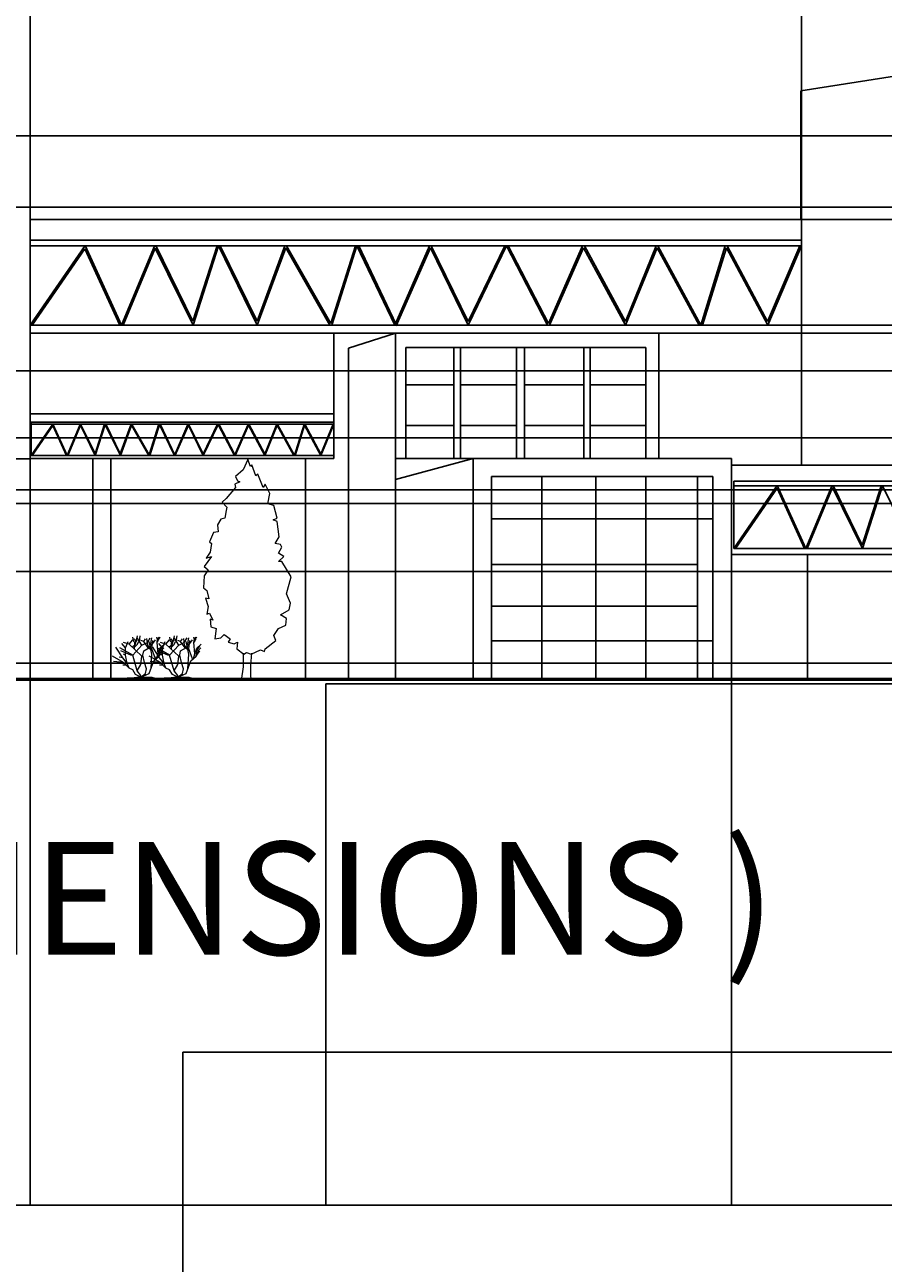
# Model space of a CAD drawing. Units: inches. Extents: x -32109 to 33221, y -19197 to 7608.
# Tile 18 of 25: x 6939 to 12337, y -5795 to 1998. Entities that reach past the tile are written whole.
import ezdxf

# ---------------------------------------------------------------- set-up
doc = ezdxf.new("R2010")
doc.units = ezdxf.units.IN
doc.header["$MEASUREMENT"] = 0
for name, color, linetype, lineweight in [('A-ANNO-DIMS', 2, 'Continuous', 18), ('A-ANNO-TEXT', 7, 'Continuous', 25), ('A-ELEV', 7, 'Continuous', 25), ('L-PLNT', 3, 'Continuous', 13)]:
    doc.layers.add(name, color=color, linetype=linetype, lineweight=lineweight)
doc.styles.get("Standard").update_dxf_attribs({"font": 'arial.ttf'})
doc.dimstyles.get("Standard").update_dxf_attribs({"dimtxt": 0.18, "dimasz": 0.18, "dimexe": 0.18, "dimexo": 0.0625, "dimgap": 0.09, "dimtad": 0, "dimtih": 1, "dimtoh": 1, "dimdec": 4, "dimzin": 0, "dimdsep": 46, "dimtxsty": 'Standard', "dimcen": 0.09, "dimadec": 0, "dimazin": 0, "dimtfac": 1, "dimtdec": 4, "dimtofl": 0, "dimtmove": 0, "dimatfit": 3, "dimfxl": 1, "dimtolj": 1, "dimtzin": 0, "dimarcsym": 0})

# ---------------------------------------------------------------- blocks, each defined once
blk = doc.blocks.new('*U2')
blk.add_lwpolyline([(-2.754, 191.699), (-6.78, 182.851), (-13.682, 176.953), (-11.956, 173.266), (-9.656, 172.529), (-14.257, 170.317), (-13.682, 167.368), (-21.733, 157.783), (-25.184, 154.834), (-21.158, 150.41), (-21.733, 147.461), (-22.884, 140.825), (-26.334, 140.087), (-29.21, 134.926), (-28.635, 129.028), (-32.661, 128.291), (-36.111, 120.18), (-34.386, 118.706), (-35.536, 111.333), (-38.987, 106.171), (-34.386, 107.646), (-40.712, 98.798), (-37.261, 95.849), (-40.712, 90.688), (-41.287, 80.366), (-38.412, 78.154), (-36.686, 70.781), (-39.562, 71.518), (-37.261, 64.145), (-38.412, 57.509), (-36.111, 58.247), (-33.236, 52.348), (-35.536, 53.086), (-34.961, 46.45), (-30.36, 44.975), (-31.51, 36.128), (-26.334, 36.865), (-23.459, 39.814), (-18.283, 36.128), (-20.008, 33.178), (-14.832, 31.704), (-11.956, 33.178), (-12.531, 27.28), (-6.205, 22.856), (-3.905, 24.331), (0.121, 22.856), (8.173, 26.543), (11.624, 25.068), (12.199, 27.28), (21.4, 34.653), (19.675, 39.077), (23.701, 44.975), (30.027, 47.924), (30.602, 53.823), (25.426, 56.772), (32.903, 61.196), (34.053, 67.094), (30.602, 75.205), (34.628, 89.951), (26.576, 103.222), (23.701, 103.222), (28.302, 107.646), (23.701, 110.595), (26.576, 115.756), (25.426, 117.968), (20.825, 118.706), (24.276, 124.604), (22.551, 137.876), (19.1, 139.35), (22.551, 140.825), (19.675, 151.884), (14.499, 153.359), (16.224, 162.207), (12.199, 170.317), (10.473, 167.368), (5.872, 179.165), (4.147, 177.69), (0.696, 187.275), (-0.454, 185.8)], close=True)
for points in [[(-6.813, 23.669), (-6.813, 11.669), (-8.627, 0)], [(0.387, 23.669), (-0.576, 13.271), (-0.576, 3.686), (0, 0)]]:
    blk.add_lwpolyline(points)
blk = doc.blocks.new('*U3')
for p, q in [((-16.8, 16.32), (-15.36, 19.68)), ((-14.88, 18.24), (-12.96, 20.64)), ((-12.471, 19.775), (-12.898, 22.044)), ((-11.677, 19.071), (-12.471, 19.775)), ((-11.28, 19.619), (-12.104, 21.184)), ((-11.921, 18.836), (-10.64, 20.401)), ((-11.433, 18.289), (-10.457, 22.749)), ((-10.579, 18.054), (-9.846, 19.697)), ((-8.16, 17.76), (-10.56, 21.6)), ((-9.48, 19.775), (-8.992, 22.592)), ((-7.2, 19.68), (-8.64, 20.16)), ((-7.2, 19.68), (-6.24, 21.12)), ((-4.8, 16.32), (-7.2, 19.68)), ((-5.086, 17.741), (-5.513, 21.34)), ((-5.28, 19.2), (-3.84, 21.6)), ((-2.88, 12.96), (-4.32, 19.68)), ((-3.84, 16.8), (-0.96, 20.64)), ((-3.377, 18.602), (-2.888, 21.575)), ((-2.88, 15.84), (-2.4, 20.16)), ((-0.508, 21.888), (-0.081, 20.558)), ((-0.203, 19.149), (0.102, 21.34)), ((-0.142, 19.384), (0.59, 20.401)), ((-0.02, 20.01), (0.896, 21.105)), ((0.041, 20.714), (1.384, 22.044)), ((0.102, 21.34), (0.835, 21.888)), ((-18.24, 11.04), (-21.755, 16.655)), ((-12.96, 12.48), (-19.68, 16.32)), ((-13.92, 12.48), (-19.2, 14.88)), ((-16.8, 16.32), (-18.72, 18.72)), ((-14.88, 18.24), (-17.76, 19.2)), ((-16.8, 12.48), (-16.8, 16.32)), ((-8.16, 12), (-14.88, 18.24)), ((-13.325, 16.724), (-11.433, 18.289)), ((-12.96, 12.48), (-8.16, 17.76)), ((-12.043, 15.628), (-11.921, 18.836)), ((-11.982, 16.802), (-10.579, 18.054)), ((-8.16, 17.76), (-5.28, 19.2)), ((-7.68, 12.48), (-7.2, 14.88)), ((-7.2, 14.88), (-3.84, 16.8)), ((-3.377, 15.315), (-5.086, 17.819)), ((-2.766, 16.802), (-3.377, 18.602)), ((-0.96, 10.56), (-2.88, 15.84)), ((-0.48, 10.8), (0.346, 13.203)), ((0.346, 13.203), (-0.203, 19.149)), ((0.346, 13.203), (1.323, 16.254)), ((0.96, 12), (1.44, 15.36)), ((0.96, 12), (2.88, 14.88)), ((1.323, 16.254), (3.642, 18.289)), ((1.44, 15.36), (2.88, 17.28)), ((1.92, 13.44), (2.4, 15.36)), ((2.4, 15.36), (3.36, 16.32)), ((-17.76, 8.64), (-23.663, 11.961)), ((-17.76, 8.64), (-23.128, 9.222)), ((-18.24, 11.04), (-20.16, 11.52)), ((-15.84, 8.16), (-18.24, 11.04)), ((-16.32, 7.2), (-18.24, 7.2)), ((-16.8, 12.48), (-17.76, 12.96)), ((-14.88, 5.76), (-17.76, 8.64)), ((-15.84, 8.16), (-16.8, 12.48)), ((-14.88, 5.76), (-15.84, 8.16)), ((-12.96, 12.48), (-13.92, 12.48)), ((-10.56, 4.32), (-12.96, 12.48)), ((-10.56, 4.32), (-8.64, 7.68)), ((-8.64, 7.68), (-8.16, 12)), ((-6.72, 8.64), (-7.68, 12.48)), ((-5.76, 5.28), (-6.72, 8.64)), ((-4.32, 2.88), (-1.92, 9.6)), ((-3.36, 5.28), (-2.88, 12.96)), ((-1.92, 9.6), (0.96, 12)), ((-15.84, 0.48), (-17.76, 0)), ((-13.44, 0.48), (-15.84, 0.48)), ((-12.96, 4.8), (-14.88, 5.76)), ((-9.6, 0.96), (-13.44, 0.48)), ((-11.52, 2.4), (-12.96, 4.8)), ((-9.6, 0.96), (-12.96, 0)), ((-8.64, 0.96), (-11.52, 2.4)), ((-8.64, 1.92), (-10.56, 4.32)), ((-9.6, 0.96), (-7.68, 0.96)), ((-8.64, 0.96), (-4.32, 2.88)), ((-8.64, 0.96), (-6.24, 2.88)), ((-8.64, 0.96), (-8.64, 1.92)), ((-8.64, 0.96), (-2.88, 0.96)), ((-7.68, 0.96), (-6.24, 0.48)), ((-6.24, 2.88), (-5.76, 5.28)), ((-6.24, 0.48), (-3.36, 0)), ((-2.88, 0.96), (0, 0))]:
    blk.add_line(p, q)
blk = doc.blocks.new('*D10')
at = {"layer": 'A-ANNO-DIMS', "color": 0, "lineweight": -2, "transparency": 16777216}
for p, q in [((-18512.6, -110.2), (-18512.6, 5772)), ((-18512.5, 5771.8), (-202.1, 5771.8)), ((18109.1, 5771.8), (-201.2, 5771.8)), ((18109.3, -101.5), (18109.3, 5772))]:
    blk.add_line(p, q, dxfattribs=at)
at = {"layer": 'A-ANNO-DIMS', "color": 0, "transparency": 16777216}
for points in [[(-18512.5, 5771.9), (-18512.5, 5771.8), (-18512.6, 5771.8)], [(18109.1, 5771.9), (18109.1, 5771.8), (18109.3, 5771.8)]]:
    blk.add_solid(points, dxfattribs=at)
at = {"layer": 'Defpoints', "color": 0, "transparency": 16777216}
for p in [(18109.3, 5771.8), (-18512.6, -110.2), (18109.3, -101.6)]:
    blk.add_point(p, dxfattribs=at)
at = {"layer": 'A-ANNO-DIMS', "color": 0, "transparency": 16777216, "insert": (-201.7, 5771.8), "char_height": 0.18, "attachment_point": 5}
blk.add_mtext('\\A1;36622', dxfattribs=at)
blk = doc.blocks.new('*D11')
at = {"layer": 'A-ANNO-DIMS', "color": 0, "lineweight": -2, "transparency": 16777216}
for p, q in [((14509.6, 1705.2), (25710.6, 1705.2)), ((25710.5, 1705), (25710.5, -209.6)), ((25710.5, -2124.6), (25710.5, -210)), ((-18512.6, -2124.8), (25710.6, -2124.8))]:
    blk.add_line(p, q, dxfattribs=at)
at = {"layer": 'A-ANNO-DIMS', "color": 0, "transparency": 16777216}
for points in [[(25710.4, 1705), (25710.5, 1705), (25710.5, 1705.2)], [(25710.4, -2124.6), (25710.5, -2124.6), (25710.5, -2124.8)]]:
    blk.add_solid(points, dxfattribs=at)
at = {"layer": 'Defpoints', "color": 0, "transparency": 16777216}
for p in [(14509.6, 1705.2), (-18512.6, -2124.8), (25710.5, -2124.8)]:
    blk.add_point(p, dxfattribs=at)
at = {"layer": 'A-ANNO-DIMS', "color": 0, "transparency": 16777216, "insert": (25710.5, -209.8), "char_height": 0.18, "attachment_point": 5}
blk.add_mtext('\\A1;3830', dxfattribs=at)
blk = doc.blocks.new('*D16')
at = {"layer": 'A-ANNO-DIMS', "color": 0, "lineweight": -2, "transparency": 16777216}
for p, q in [((7931.9, -8929), (7931.9, -4467.1)), ((7932, -4467.3), (18774.7, -4467.3)), ((29618.2, -4467.3), (18775.5, -4467.3)), ((29618.3, -6090.7), (29618.3, -4467.1))]:
    blk.add_line(p, q, dxfattribs=at)
at = {"layer": 'A-ANNO-DIMS', "color": 0, "transparency": 16777216}
for points in [[(7932, -4467.2), (7932, -4467.3), (7931.9, -4467.3)], [(29618.2, -4467.2), (29618.2, -4467.3), (29618.3, -4467.3)]]:
    blk.add_solid(points, dxfattribs=at)
at = {"layer": 'Defpoints', "color": 0, "transparency": 16777216}
for p in [(29618.3, -4467.3), (29618.3, -6090.8), (7931.9, -8929.1)]:
    blk.add_point(p, dxfattribs=at)
at = {"layer": 'A-ANNO-DIMS', "color": 0, "transparency": 16777216, "insert": (18775.1, -4467.3), "char_height": 0.18, "attachment_point": 5}
blk.add_mtext('\\A1;21686', dxfattribs=at)
blk = doc.blocks.new('*D53')
at = {"layer": 'A-ANNO-DIMS', "color": 0, "lineweight": -2, "transparency": 16777216}
for p, q in [((-9508.3, -179.7), (25710.6, -179.7)), ((25710.5, -179.9), (25710.5, -389.7)), ((25710.5, -600), (25710.5, -390.1)), ((-9508.3, -600.2), (25710.6, -600.2))]:
    blk.add_line(p, q, dxfattribs=at)
at = {"layer": 'A-ANNO-DIMS', "color": 0, "transparency": 16777216}
for points in [[(25710.4, -179.9), (25710.5, -179.9), (25710.5, -179.7)], [(25710.4, -600), (25710.5, -600), (25710.5, -600.2)]]:
    blk.add_solid(points, dxfattribs=at)
at = {"layer": 'Defpoints', "color": 0, "transparency": 16777216}
for p in [(-9508.3, -179.7), (-9508.3, -600.2), (25710.5, -600.2)]:
    blk.add_point(p, dxfattribs=at)
at = {"layer": 'A-ANNO-DIMS', "color": 0, "transparency": 16777216, "insert": (25710.5, -389.9), "char_height": 0.18, "attachment_point": 5}
blk.add_mtext('\\A1;420.5', dxfattribs=at)
blk = doc.blocks.new('*D54')
at = {"layer": 'A-ANNO-DIMS', "color": 0, "lineweight": -2, "transparency": 16777216}
for p, q in [((-9508.3, -600.2), (25710.6, -600.2)), ((25710.5, -600.3), (25710.5, -806.8)), ((25710.5, -1013.7), (25710.5, -807.2)), ((-9508.3, -1013.9), (25710.6, -1013.9))]:
    blk.add_line(p, q, dxfattribs=at)
at = {"layer": 'A-ANNO-DIMS', "color": 0, "transparency": 16777216}
for points in [[(25710.4, -600.3), (25710.5, -600.3), (25710.5, -600.2)], [(25710.4, -1013.7), (25710.5, -1013.7), (25710.5, -1013.9)]]:
    blk.add_solid(points, dxfattribs=at)
at = {"layer": 'Defpoints', "color": 0, "transparency": 16777216}
for p in [(-9508.3, -600.2), (-9508.3, -1013.9), (25710.5, -1013.9)]:
    blk.add_point(p, dxfattribs=at)
at = {"layer": 'A-ANNO-DIMS', "color": 0, "transparency": 16777216, "insert": (25710.5, -807), "char_height": 0.18, "attachment_point": 5}
blk.add_mtext('\\A1;413.7', dxfattribs=at)
blk = doc.blocks.new('*D55')
at = {"layer": 'A-ANNO-DIMS', "color": 0, "lineweight": -2, "transparency": 16777216}
for p, q in [((-9508.3, -1013.9), (25710.6, -1013.9)), ((25710.5, -1014.1), (25710.5, -1227.7)), ((25710.5, -1441.6), (25710.5, -1228)), ((-9508.3, -1441.8), (25710.6, -1441.8))]:
    blk.add_line(p, q, dxfattribs=at)
at = {"layer": 'A-ANNO-DIMS', "color": 0, "transparency": 16777216}
for points in [[(25710.4, -1014.1), (25710.5, -1014.1), (25710.5, -1013.9)], [(25710.4, -1441.6), (25710.5, -1441.6), (25710.5, -1441.8)]]:
    blk.add_solid(points, dxfattribs=at)
at = {"layer": 'Defpoints', "color": 0, "transparency": 16777216}
for p in [(-9508.3, -1013.9), (-9508.3, -1441.8), (25710.5, -1441.8)]:
    blk.add_point(p, dxfattribs=at)
at = {"layer": 'A-ANNO-DIMS', "color": 0, "transparency": 16777216, "insert": (25710.5, -1227.9), "char_height": 0.18, "attachment_point": 5}
blk.add_mtext('\\A1;427.9', dxfattribs=at)
blk = doc.blocks.new('*D56')
at = {"layer": 'A-ANNO-DIMS', "color": 0, "lineweight": -2, "transparency": 16777216}
for p, q in [((-9508.3, -1441.8), (25710.6, -1441.8)), ((25710.5, -1442), (25710.5, -1730.1)), ((25710.5, -2018.6), (25710.5, -1730.5)), ((-9508.3, -2018.8), (25710.6, -2018.8))]:
    blk.add_line(p, q, dxfattribs=at)
at = {"layer": 'A-ANNO-DIMS', "color": 0, "transparency": 16777216}
for points in [[(25710.4, -1442), (25710.5, -1442), (25710.5, -1441.8)], [(25710.4, -2018.6), (25710.5, -2018.6), (25710.5, -2018.8)]]:
    blk.add_solid(points, dxfattribs=at)
at = {"layer": 'Defpoints', "color": 0, "transparency": 16777216}
for p in [(-9508.3, -1441.8), (-9508.3, -2018.8), (25710.5, -2018.8)]:
    blk.add_point(p, dxfattribs=at)
at = {"layer": 'A-ANNO-DIMS', "color": 0, "transparency": 16777216, "insert": (25710.5, -1730.3), "char_height": 0.18, "attachment_point": 5}
blk.add_mtext('\\A1;576.9', dxfattribs=at)
blk = doc.blocks.new('*D59')
at = {"layer": 'A-ANNO-DIMS', "color": 0, "lineweight": -2, "transparency": 16777216}
for p, q in [((6972.5, 1298.6), (6972.5, -5429.7)), ((5279.3, -2122.8), (5279.3, -5429.7)), ((5279.4, -5429.6), (6125.5, -5429.6)), ((6972.4, -5429.6), (6126.4, -5429.6))]:
    blk.add_line(p, q, dxfattribs=at)
at = {"layer": 'A-ANNO-DIMS', "color": 0, "transparency": 16777216}
for points in [[(5279.4, -5429.5), (5279.4, -5429.6), (5279.3, -5429.6)], [(6972.4, -5429.5), (6972.4, -5429.6), (6972.5, -5429.6)]]:
    blk.add_solid(points, dxfattribs=at)
at = {"layer": 'Defpoints', "color": 0, "transparency": 16777216}
for p in [(6972.5, 1298.7), (5279.3, -2122.7), (6972.5, -5429.6)]:
    blk.add_point(p, dxfattribs=at)
at = {"layer": 'A-ANNO-DIMS', "color": 0, "transparency": 16777216, "insert": (6125.9, -5429.6), "char_height": 0.18, "attachment_point": 5}
blk.add_mtext('\\A1;1693.3', dxfattribs=at)
blk = doc.blocks.new('*D60')
at = {"layer": 'A-ANNO-DIMS', "color": 0, "lineweight": -2, "transparency": 16777216}
for p, q in [((6972.5, 1298.6), (6972.5, -5429.7)), ((8832.3, -2148.4), (8832.3, -5429.7)), ((6972.7, -5429.6), (7902, -5429.6)), ((8832.1, -5429.6), (7902.9, -5429.6))]:
    blk.add_line(p, q, dxfattribs=at)
at = {"layer": 'A-ANNO-DIMS', "color": 0, "transparency": 16777216}
for points in [[(6972.7, -5429.5), (6972.7, -5429.6), (6972.5, -5429.6)], [(8832.1, -5429.5), (8832.1, -5429.6), (8832.3, -5429.6)]]:
    blk.add_solid(points, dxfattribs=at)
at = {"layer": 'Defpoints', "color": 0, "transparency": 16777216}
for p in [(6972.5, 1298.7), (8832.3, -2148.4), (8832.3, -5429.6)]:
    blk.add_point(p, dxfattribs=at)
at = {"layer": 'A-ANNO-DIMS', "color": 0, "transparency": 16777216, "insert": (7902.4, -5429.6), "char_height": 0.18, "attachment_point": 5}
blk.add_mtext('\\A1;1859.7', dxfattribs=at)
blk = doc.blocks.new('*D61')
at = {"layer": 'A-ANNO-DIMS', "color": 0, "lineweight": -2, "transparency": 16777216}
for p, q in [((8832.3, -2148.4), (8832.3, -5429.7)), ((11383.7, -2116.2), (11383.7, -5429.7)), ((8832.5, -5429.6), (10107.5, -5429.6)), ((11383.5, -5429.6), (10108.5, -5429.6))]:
    blk.add_line(p, q, dxfattribs=at)
at = {"layer": 'A-ANNO-DIMS', "color": 0, "transparency": 16777216}
for points in [[(8832.5, -5429.5), (8832.5, -5429.6), (8832.3, -5429.6)], [(11383.5, -5429.5), (11383.5, -5429.6), (11383.7, -5429.6)]]:
    blk.add_solid(points, dxfattribs=at)
at = {"layer": 'Defpoints', "color": 0, "transparency": 16777216}
for p in [(8832.3, -2148.4), (11383.7, -2116.1), (11383.7, -5429.6)]:
    blk.add_point(p, dxfattribs=at)
at = {"layer": 'A-ANNO-DIMS', "color": 0, "transparency": 16777216, "insert": (10108, -5429.6), "char_height": 0.18, "attachment_point": 5}
blk.add_mtext('\\A1;2551.4', dxfattribs=at)
blk = doc.blocks.new('*D62')
at = {"layer": 'A-ANNO-DIMS', "color": 0, "lineweight": -2, "transparency": 16777216}
for p, q in [((12596.6, 1705.1), (12596.6, -5429.7)), ((11383.7, -2116.2), (11383.7, -5429.7)), ((11383.9, -5429.6), (11989.8, -5429.6)), ((12596.5, -5429.6), (11990.5, -5429.6))]:
    blk.add_line(p, q, dxfattribs=at)
at = {"layer": 'A-ANNO-DIMS', "color": 0, "transparency": 16777216}
for points in [[(11383.9, -5429.5), (11383.9, -5429.6), (11383.7, -5429.6)], [(12596.5, -5429.5), (12596.5, -5429.6), (12596.6, -5429.6)]]:
    blk.add_solid(points, dxfattribs=at)
at = {"layer": 'Defpoints', "color": 0, "transparency": 16777216}
for p in [(12596.6, 1705.2), (11383.7, -2116.1), (12596.6, -5429.6)]:
    blk.add_point(p, dxfattribs=at)
at = {"layer": 'A-ANNO-DIMS', "color": 0, "transparency": 16777216, "insert": (11990.2, -5429.6), "char_height": 0.18, "attachment_point": 5}
blk.add_mtext('\\A1;1213', dxfattribs=at)
blk = doc.blocks.new('*D67')
at = {"layer": 'A-ANNO-DIMS', "color": 0, "lineweight": -2, "transparency": 16777216}
for p, q in [((1645.9, 851.2), (25710.6, 851.2)), ((25710.5, 851), (25710.5, -632.3)), ((25710.5, -2116), (25710.5, -632.7)), ((1588.2, -2116.1), (25710.6, -2116.1))]:
    blk.add_line(p, q, dxfattribs=at)
at = {"layer": 'A-ANNO-DIMS', "color": 0, "transparency": 16777216}
for points in [[(25710.4, 851), (25710.5, 851), (25710.5, 851.2)], [(25710.4, -2116), (25710.5, -2116), (25710.5, -2116.1)]]:
    blk.add_solid(points, dxfattribs=at)
at = {"layer": 'Defpoints', "color": 0, "transparency": 16777216}
for p in [(1645.8, 851.2), (1588.2, -2116.1), (25710.5, -2116.1)]:
    blk.add_point(p, dxfattribs=at)
at = {"layer": 'A-ANNO-DIMS', "color": 0, "transparency": 16777216, "insert": (25710.5, -632.5), "char_height": 0.18, "attachment_point": 5}
blk.add_mtext('\\A1;2967.4', dxfattribs=at)
blk = doc.blocks.new('*D68')
at = {"layer": 'A-ANNO-DIMS', "color": 0, "lineweight": -2, "transparency": 16777216}
for p, q in [((4084.1, -927.5), (25710.6, -927.5)), ((25710.5, -927.7), (25710.5, -1521.6)), ((25710.5, -2116), (25710.5, -1522)), ((4084.1, -2116.1), (25710.6, -2116.1))]:
    blk.add_line(p, q, dxfattribs=at)
at = {"layer": 'A-ANNO-DIMS', "color": 0, "transparency": 16777216}
for points in [[(25710.4, -927.7), (25710.5, -927.7), (25710.5, -927.5)], [(25710.4, -2116), (25710.5, -2116), (25710.5, -2116.1)]]:
    blk.add_solid(points, dxfattribs=at)
at = {"layer": 'Defpoints', "color": 0, "transparency": 16777216}
for p in [(4084, -927.5), (4084, -2116.1), (25710.5, -2116.1)]:
    blk.add_point(p, dxfattribs=at)
at = {"layer": 'A-ANNO-DIMS', "color": 0, "transparency": 16777216, "insert": (25710.5, -1521.8), "char_height": 0.18, "attachment_point": 5}
blk.add_mtext('\\A1;1188.7', dxfattribs=at)
blk = doc.blocks.new('*D69')
at = {"layer": 'A-ANNO-DIMS', "color": 0, "lineweight": -2, "transparency": 16777216}
for p, q in [((5273.8, 1298.7), (25710.6, 1298.7)), ((25710.5, 1298.5), (25710.5, -411.9)), ((25710.5, -2122.6), (25710.5, -412.2)), ((5279.3, -2122.7), (25710.6, -2122.7))]:
    blk.add_line(p, q, dxfattribs=at)
at = {"layer": 'A-ANNO-DIMS', "color": 0, "transparency": 16777216}
for points in [[(25710.4, 1298.5), (25710.5, 1298.5), (25710.5, 1298.7)], [(25710.4, -2122.6), (25710.5, -2122.6), (25710.5, -2122.7)]]:
    blk.add_solid(points, dxfattribs=at)
at = {"layer": 'Defpoints', "color": 0, "transparency": 16777216}
for p in [(5273.7, 1298.7), (5279.3, -2122.7), (25710.5, -2122.7)]:
    blk.add_point(p, dxfattribs=at)
at = {"layer": 'A-ANNO-DIMS', "color": 0, "transparency": 16777216, "insert": (25710.5, -412), "char_height": 0.18, "attachment_point": 5}
blk.add_mtext('\\A1;3421.4', dxfattribs=at)
blk = doc.blocks.new('*D70')
at = {"layer": 'A-ANNO-DIMS', "color": 0, "lineweight": -2, "transparency": 16777216}
for p, q in [((8883.3, 57.8), (25710.6, 57.8)), ((25710.5, 57.6), (25710.5, -1045.1)), ((25710.5, -2148.2), (25710.5, -1045.5)), ((8832.4, -2148.4), (25710.6, -2148.4))]:
    blk.add_line(p, q, dxfattribs=at)
at = {"layer": 'A-ANNO-DIMS', "color": 0, "transparency": 16777216}
for points in [[(25710.4, 57.6), (25710.5, 57.6), (25710.5, 57.8)], [(25710.4, -2148.2), (25710.5, -2148.2), (25710.5, -2148.4)]]:
    blk.add_solid(points, dxfattribs=at)
at = {"layer": 'Defpoints', "color": 0, "transparency": 16777216}
for p in [(8883.2, 57.8), (8832.3, -2148.4), (25710.5, -2148.4)]:
    blk.add_point(p, dxfattribs=at)
at = {"layer": 'A-ANNO-DIMS', "color": 0, "transparency": 16777216, "insert": (25710.5, -1045.3), "char_height": 0.18, "attachment_point": 5}
blk.add_mtext('\\A1;2206', dxfattribs=at)
blk = doc.blocks.new('*D71')
at = {"layer": 'A-ANNO-DIMS', "color": 0, "lineweight": -2, "transparency": 16777216}
for p, q in [((11823.3, 772.8), (25710.6, 772.8)), ((25710.5, 772.6), (25710.5, 440.5)), ((25710.5, 107.9), (25710.5, 440.1)), ((11823.3, 107.7), (25710.6, 107.7))]:
    blk.add_line(p, q, dxfattribs=at)
at = {"layer": 'A-ANNO-DIMS', "color": 0, "transparency": 16777216}
for points in [[(25710.4, 772.6), (25710.5, 772.6), (25710.5, 772.8)], [(25710.4, 107.9), (25710.5, 107.9), (25710.5, 107.7)]]:
    blk.add_solid(points, dxfattribs=at)
at = {"layer": 'Defpoints', "color": 0, "transparency": 16777216}
for p in [(11823.2, 772.8), (11823.2, 107.7), (25710.5, 107.7)]:
    blk.add_point(p, dxfattribs=at)
at = {"layer": 'A-ANNO-DIMS', "color": 0, "transparency": 16777216, "insert": (25710.5, 440.3), "char_height": 0.18, "attachment_point": 5}
blk.add_mtext('\\A1;665.1', dxfattribs=at)
blk = doc.blocks.new('*D72')
at = {"layer": 'A-ANNO-DIMS', "color": 0, "lineweight": -2, "transparency": 16777216}
for p, q in [((11823.3, 107.7), (25710.6, 107.7)), ((25710.5, 107.6), (25710.5, -1004)), ((25710.5, -2116), (25710.5, -1004.4)), ((11383.7, -2116.1), (25710.6, -2116.1))]:
    blk.add_line(p, q, dxfattribs=at)
at = {"layer": 'A-ANNO-DIMS', "color": 0, "transparency": 16777216}
for points in [[(25710.4, 107.6), (25710.5, 107.6), (25710.5, 107.7)], [(25710.4, -2116), (25710.5, -2116), (25710.5, -2116.1)]]:
    blk.add_solid(points, dxfattribs=at)
at = {"layer": 'Defpoints', "color": 0, "transparency": 16777216}
for p in [(11823.2, 107.7), (11383.7, -2116.1), (25710.5, -2116.1)]:
    blk.add_point(p, dxfattribs=at)
at = {"layer": 'A-ANNO-DIMS', "color": 0, "transparency": 16777216, "insert": (25710.5, -1004.2), "char_height": 0.18, "attachment_point": 5}
blk.add_mtext('\\A1;2224', dxfattribs=at)
blk = doc.blocks.new('*D73')
at = {"layer": 'A-ANNO-DIMS', "color": 0, "lineweight": -2, "transparency": 16777216}
for p, q in [((6972.5, 772.9), (6972.5, 5772)), ((6972.7, 5771.8), (9397.5, 5771.8)), ((11823.1, 5771.8), (9398.2, 5771.8)), ((11823.2, 772.9), (11823.2, 5772))]:
    blk.add_line(p, q, dxfattribs=at)
at = {"layer": 'A-ANNO-DIMS', "color": 0, "transparency": 16777216}
for points in [[(6972.7, 5771.9), (6972.7, 5771.8), (6972.5, 5771.8)], [(11823.1, 5771.9), (11823.1, 5771.8), (11823.2, 5771.8)]]:
    blk.add_solid(points, dxfattribs=at)
at = {"layer": 'Defpoints', "color": 0, "transparency": 16777216}
for p in [(11823.2, 5771.8), (6972.5, 772.8), (11823.2, 772.8)]:
    blk.add_point(p, dxfattribs=at)
at = {"layer": 'A-ANNO-DIMS', "color": 0, "transparency": 16777216, "insert": (9397.9, 5771.8), "char_height": 0.18, "attachment_point": 5}
blk.add_mtext('\\A1;4851', dxfattribs=at)

msp = doc.modelspace()

# ---------------------------------------------------------------- linework, layer by layer
at = {"layer": 'A-ELEV'}
for p, q in [((11819.608, 1582.37), (12596.642, 1705.162)), ((11819.608, 772.828), (11819.608, 1582.37)), ((5273.749, 1298.671), (6972.548, 1298.671)), ((6972.548, 1298.671), (6972.548, -732.655)), ((6972.548, 772.828), (11823.239, 772.828)), ((11823.239, 772.828), (11823.239, 643.904)), ((11823.239, 643.904), (6972.548, 643.904)), ((6972.548, 107.745), (6972.548, 643.904)), ((11823.239, 607.565), (11823.239, 643.904)), ((6972.548, 107.745), (7318.526, 609.489)), ((6972.548, 607.565), (11823.239, 607.565)), ((6984.694, 107.745), (7316.737, 589.278)), ((7316.737, 589.278), (7535.877, 107.745)), ((7318.526, 609.489), (7546.939, 107.58)), ((7546.939, 107.58), (7753.939, 605.211)), ((7557.839, 107.745), (7759.8, 593.264)), ((7759.8, 593.264), (7998.057, 107.58)), ((7762.917, 609.615), (7996.105, 134.264)), ((7996.105, 134.264), (8147.743, 607.565)), ((7998.057, 107.58), (8157.946, 606.637)), ((8157.946, 606.637), (8400.636, 107.58)), ((8168.615, 607.565), (8399.388, 133.012)), ((8399.388, 133.012), (8575.067, 607.565)), ((8400.636, 107.58), (8580.81, 594.273)), ((8580.81, 594.273), (8856.978, 107.745)), ((8585.349, 606.534), (8862.706, 117.913)), ((8862.706, 117.913), (9017.777, 607.565)), ((8869.975, 107.745), (9028.055, 606.897)), ((9028.055, 606.897), (9265.41, 107.485)), ((9038.809, 607.565), (9274.441, 111.778)), ((9265.41, 107.485), (9483.984, 606.83)), ((9274.57, 103.476), (9489.729, 595.017)), ((9489.729, 595.017), (9726.872, 107.427)), ((9494.747, 607.565), (9726.848, 130.339)), ((9726.848, 130.339), (9957.748, 607.565)), ((9726.872, 107.427), (9968.446, 606.717)), ((9968.446, 606.717), (10226.994, 107.375)), ((9979.268, 607.565), (10232.173, 119.122)), ((10232.173, 119.122), (10447.091, 606.639)), ((10238.086, 107.745), (10453.111, 595.505)), ((10453.111, 595.505), (10717.03, 107.361)), ((10457.958, 607.565), (10715.745, 130.764)), ((10715.745, 130.764), (10909.46, 607.565)), ((10717.03, 107.361), (10915.075, 594.819)), ((10915.075, 594.819), (11179.752, 107.745)), ((10919.944, 606.803), (11191.296, 107.447)), ((11191.296, 107.447), (11344.222, 606.875)), ((11201.846, 107.745), (11350.873, 594.439)), ((11350.873, 594.439), (11611.354, 107.397)), ((11355.193, 607.565), (11610.304, 130.563)), ((11610.304, 130.563), (11812.306, 607.565)), ((11611.354, 107.397), (11823.239, 607.739)), ((11823.239, 607.565), (11823.239, 107.745)), ((11823.239, 107.745), (6972.548, 107.745)), ((10226.994, 107.375), (10227.157, 107.745)), ((11823.239, 57.799), (11823.239, 107.745)), ((6972.548, 57.799), (11823.239, 57.799)), ((8883.215, -450.892), (8883.215, 57.799)), ((8883.215, 57.799), (10926.233, 57.799)), ((9270.543, 57.799), (8975.053, -36.902)), ((9270.543, -731.481), (9270.543, 57.799)), ((10926.233, 57.799), (10926.233, -731.481)), ((11823.239, -13.943), (11823.239, 57.799)), ((8975.053, -36.902), (8975.053, -731.481)), ((9335.51, -731.481), (9335.51, -33.368)), ((9335.51, -33.368), (10844.686, -33.368)), ((9636.73, -731.481), (9636.73, -33.368)), ((9679.219, -731.481), (9679.219, -33.368)), ((10031.696, -731.481), (10031.696, -33.368)), ((10080.967, -731.481), (10080.967, -33.368)), ((10455.429, -731.481), (10455.429, -33.368)), ((10494.846, -731.481), (10494.846, -33.368)), ((10844.686, -33.368), (10844.686, -731.481)), ((11823.239, -101.6), (11823.239, -13.943)), ((11823.239, -101.6), (11823.239, -771.886)), ((9335.51, -267.245), (9636.73, -267.245)), ((9679.219, -267.245), (10031.696, -267.245)), ((10080.967, -267.245), (10455.429, -267.245)), ((10494.846, -267.245), (10844.686, -267.245)), ((6972.548, -450.892), (8883.215, -450.892)), ((8883.215, -450.892), (8883.215, -501.484)), ((8883.215, -501.484), (6979.723, -501.484)), ((6979.723, -711.881), (6979.723, -501.484)), ((6979.723, -711.881), (7115.49, -514.989)), ((6979.723, -515.744), (8883.215, -515.744)), ((6984.489, -711.881), (7114.788, -522.92)), ((7114.788, -522.92), (7200.783, -711.881)), ((7115.49, -514.989), (7205.124, -711.946)), ((7205.124, -711.946), (7286.354, -516.668)), ((7209.401, -711.881), (7288.654, -521.356)), ((7288.654, -521.356), (7382.149, -711.946)), ((7289.877, -514.939), (7381.384, -701.475)), ((7381.384, -701.475), (7440.889, -515.744)), ((7382.149, -711.946), (7444.893, -516.108)), ((7444.893, -516.108), (7540.128, -711.946)), ((7449.079, -515.744), (7539.639, -701.966)), ((7539.639, -701.966), (7608.578, -515.744)), ((7540.128, -711.946), (7610.832, -520.96)), ((7610.832, -520.96), (7719.205, -711.881)), ((7612.613, -516.148), (7721.452, -707.891)), ((7721.452, -707.891), (7782.305, -515.744)), ((7724.305, -711.881), (7786.338, -516.006)), ((7786.338, -516.006), (7879.48, -711.983)), ((7790.558, -515.744), (7883.024, -710.299)), ((7879.48, -711.983), (7965.252, -516.032)), ((7883.075, -713.557), (7967.507, -520.668)), ((7967.507, -520.668), (8060.565, -712.006)), ((7969.476, -515.744), (8060.556, -703.015)), ((8060.556, -703.015), (8151.165, -515.744)), ((8060.565, -712.006), (8155.363, -516.077)), ((8155.363, -516.077), (8256.822, -712.027)), ((8159.61, -515.744), (8258.854, -707.417)), ((8258.854, -707.417), (8343.192, -516.107)), ((8261.175, -711.881), (8345.554, -520.476)), ((8345.554, -520.476), (8449.12, -712.032)), ((8347.456, -515.744), (8448.616, -702.848)), ((8448.616, -702.848), (8524.633, -515.744)), ((8449.12, -712.032), (8526.837, -520.746)), ((8526.837, -520.746), (8630.7, -711.881)), ((8528.747, -516.043), (8635.23, -711.999)), ((8635.23, -711.999), (8695.241, -516.015)), ((8639.37, -711.881), (8697.851, -520.894)), ((8697.851, -520.894), (8800.068, -712.018)), ((8699.546, -515.744), (8799.656, -702.927)), ((8799.656, -702.927), (8878.925, -515.744)), ((8800.068, -712.018), (8883.215, -515.676)), ((8883.215, -515.744), (8883.215, -501.484)), ((8883.215, -515.744), (8883.215, -711.881)), ((9335.51, -524.136), (9636.73, -524.136)), ((9679.219, -524.136), (10031.696, -524.136)), ((10080.967, -524.136), (10455.429, -524.136)), ((10494.846, -524.136), (10844.686, -524.136)), ((5928.838, -732.655), (6972.548, -732.655)), ((6972.548, -731.481), (8883.215, -731.481)), ((8883.215, -711.881), (6979.723, -711.881)), ((7366, -731.481), (7366, -2116.149)), ((7480.051, -731.481), (7480.051, -2116.149)), ((8256.822, -712.027), (8256.886, -711.881)), ((8705.138, -731.481), (8705.138, -2116.149)), ((8883.215, -731.481), (8883.215, -711.881)), ((8975.053, -731.481), (8975.053, -2116.149)), ((9270.543, -731.481), (9759.412, -731.481)), ((9759.412, -731.481), (9270.543, -862.543)), ((9270.543, -731.481), (9270.543, -862.543)), ((9759.412, -731.481), (9759.412, -2116.149)), ((9759.412, -731.481), (11383.682, -731.481)), ((11383.682, -731.481), (11383.682, -2116.149)), ((11384.05, -771.886), (15223.17, -771.886)), ((9873.793, -2116.149), (9873.793, -844.177)), ((9873.793, -844.177), (11265.349, -844.177)), ((10190.07, -2116.149), (10190.07, -844.177)), ((10529.942, -2116.149), (10529.942, -844.177)), ((10844.831, -2116.149), (10844.831, -844.177)), ((11169.261, -2116.149), (11169.261, -844.177)), ((11265.349, -844.177), (11265.349, -2116.149)), ((9270.543, -862.543), (9270.543, -2116.149)), ((15223.17, -873.541), (11398.466, -873.541)), ((11398.466, -1296.295), (11398.466, -873.541)), ((11398.466, -1296.295), (11671.265, -900.677)), ((11398.466, -902.193), (15223.17, -902.193)), ((11408.044, -1296.295), (11669.855, -916.613)), ((11669.855, -916.613), (11842.644, -1296.295)), ((11671.265, -900.677), (11851.367, -1296.425)), ((11851.367, -1296.425), (12014.583, -904.05)), ((11859.961, -1296.295), (12019.204, -913.47)), ((12019.204, -913.47), (12207.066, -1296.425)), ((12021.662, -900.577), (12205.527, -1275.385)), ((12205.527, -1275.385), (12325.092, -902.193)), ((12207.066, -1296.425), (12333.137, -902.926)), ((12333.137, -902.926), (12524.495, -1296.425)), ((9873.793, -1111.208), (11265.349, -1111.208)), ((15223.17, -1296.295), (11398.466, -1296.295)), ((9873.793, -1398.522), (11169.261, -1398.522)), ((11384.05, -1335.677), (15223.17, -1335.677)), ((11860.567, -1335.677), (11860.567, -2116.149)), ((9873.793, -1659.232), (11169.261, -1659.232)), ((9873.793, -1877.378), (11265.349, -1877.378)), ((3034.294, -2116.149), (9873.793, -2116.149)), ((9873.793, -2116.149), (23260.469, -2116.149))]:
    msp.add_line(p, q, dxfattribs=at)

# ---------------------------------------------------------------- block references
at = {"layer": 'L-PLNT'}
for name, p, xscale, yscale, zscale in [('*U2', (8362.331, -2127.104), 7.247071498988421, 7.247071498988421, 7.247071498988421), ('*U3', (7773.073, -2118.431), 11.97885450539613, 11.97885450539613, 11.97885450539613), ('*U3', (8005.185, -2118.431), 11.97885450539613, 11.97885450539613, 11.97885450539613)]:
    msp.add_blockref(name, p, dxfattribs=dict(at, xscale=xscale, yscale=yscale, zscale=zscale))

# ---------------------------------------------------------------- texts
at = {"layer": 'A-ANNO-TEXT'}
msp.add_text('MONUMENTAL    FRONT   FACADE    ( CONCEPTUAL ONLY   NO DIMENSIONS )', height=709.79495, dxfattribs=at).set_placement((-22238.107, -3853.852))

# ---------------------------------------------------------------- dimensions: what is measured, and where the dimension line sits
at = {"layer": 'A-ANNO-DIMS'}
for base, p1, p2, override, picture, middle in [((18109.317, 5771.835), (-18512.647, -110.242), (18109.317, -101.6), {"dimdec": 0, "dimlfac": 1, "dimrnd": 0, "dimzin": 0, "dimdsep": 46, "dimlunit": 2}, '*D10', (-201.665, 5771.835)), ((11823.239, 5771.835), (6972.548, 772.828), (11823.239, 772.828), {"dimdec": 0, "dimlfac": 1, "dimrnd": 0, "dimzin": 0, "dimdsep": 46, "dimlunit": 2}, '*D73', (9397.893, 5771.835)), ((12596.642, -5429.555), (11383.682, -2116.149), (12596.642, 1705.162), {"dimdec": 0, "dimlfac": 1, "dimrnd": 0, "dimzin": 0, "dimdsep": 46, "dimlunit": 2}, '*D62', (11990.162, -5429.555)), ((6972.548, -5429.555), (5279.264, -2122.749), (6972.548, 1298.671), {"dimdec": 1, "dimlfac": 1, "dimrnd": 0, "dimzin": 0, "dimdsep": 46, "dimlunit": 2}, '*D59', (6125.906, -5429.555)), ((8832.289, -5429.555), (6972.548, 1298.671), (8832.289, -2148.367), {"dimdec": 1, "dimlfac": 1, "dimrnd": 0, "dimzin": 0, "dimdsep": 46, "dimlunit": 2}, '*D60', (7902.418, -5429.555)), ((11383.682, -5429.555), (8832.289, -2148.367), (11383.682, -2116.149), {"dimdec": 1, "dimlfac": 1, "dimrnd": 0, "dimzin": 0, "dimdsep": 46, "dimlunit": 2}, '*D61', (10107.985, -5429.555)), ((29618.33, -4467.266), (7931.857, -8929.065), (29618.33, -6090.794), {"dimdec": 0, "dimlfac": 1, "dimrnd": 0, "dimzin": 0, "dimdsep": 46, "dimlunit": 2}, '*D16', (18775.094, -4467.266))]:
    dim = msp.add_linear_dim(base=base, p1=p1, p2=p2, dimstyle='Standard', override=override, dxfattribs=at)
    dim.commit()
    dim.dimension.update_dxf_attribs({"geometry": picture, "text_midpoint": middle})
for base, p1, p2, override, picture, middle in [((25710.469, -2124.791), (14509.55, 1705.162), (-18512.647, -2124.791), {"dimdec": 0, "dimlfac": 1, "dimrnd": 0, "dimzin": 0, "dimdsep": 46, "dimlunit": 2}, '*D11', (25710.469, -209.814)), ((25710.469, -2122.749), (5273.749, 1298.671), (5279.264, -2122.749), {"dimdec": 1, "dimlfac": 1, "dimrnd": 0, "dimzin": 0, "dimdsep": 46, "dimlunit": 2}, '*D69', (25710.469, -412.039)), ((25710.469, -2116.149), (1645.845, 851.205), (1588.181, -2116.149), {"dimdec": 1, "dimlfac": 1, "dimrnd": 0, "dimzin": 0, "dimdsep": 46, "dimlunit": 2}, '*D67', (25710.469, -632.472)), ((25710.469, 107.745), (11823.239, 772.828), (11823.239, 107.745), {"dimdec": 1, "dimlfac": 1, "dimrnd": 0, "dimzin": 0, "dimdsep": 46, "dimlunit": 2}, '*D71', (25710.469, 440.287)), ((25710.469, -2116.149), (11823.239, 107.745), (11383.682, -2116.149), {"dimdec": 0, "dimlfac": 1, "dimrnd": 0, "dimzin": 0, "dimdsep": 46, "dimlunit": 2}, '*D72', (25710.469, -1004.202)), ((25710.469, -2148.367), (8883.215, 57.799), (8832.289, -2148.367), {"dimdec": 0, "dimlfac": 1, "dimrnd": 0, "dimzin": 0, "dimdsep": 46, "dimlunit": 2}, '*D70', (25710.469, -1045.284)), ((25710.469, -600.154), (-9508.333, -179.679), (-9508.333, -600.154), {"dimdec": 1, "dimlfac": 1, "dimrnd": 0, "dimzin": 0, "dimdsep": 46, "dimlunit": 2}, '*D53', (25710.469, -389.916)), ((25710.469, -1013.888), (-9508.333, -600.154), (-9508.333, -1013.888), {"dimdec": 1, "dimlfac": 1, "dimrnd": 0, "dimzin": 0, "dimdsep": 46, "dimlunit": 2}, '*D54', (25710.469, -807.021)), ((25710.469, -2116.149), (4083.997, -927.479), (4083.997, -2116.149), {"dimdec": 1, "dimlfac": 1, "dimrnd": 0, "dimzin": 0, "dimdsep": 46, "dimlunit": 2}, '*D68', (25710.469, -1521.814)), ((25710.469, -1441.815), (-9508.333, -1013.888), (-9508.333, -1441.815), {"dimdec": 1, "dimlfac": 1, "dimrnd": 0, "dimzin": 0, "dimdsep": 46, "dimlunit": 2}, '*D55', (25710.469, -1227.851)), ((25710.469, -2018.754), (-9508.333, -1441.815), (-9508.333, -2018.754), {"dimdec": 1, "dimlfac": 1, "dimrnd": 0, "dimzin": 0, "dimdsep": 46, "dimlunit": 2}, '*D56', (25710.469, -1730.285))]:
    dim = msp.add_linear_dim(base=base, p1=p1, p2=p2, angle=90, dimstyle='Standard', override=override, dxfattribs=at)
    dim.commit()
    dim.dimension.update_dxf_attribs({"geometry": picture, "text_midpoint": middle})

doc.saveas('drawing.dxf')
